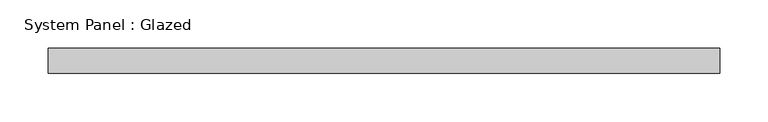
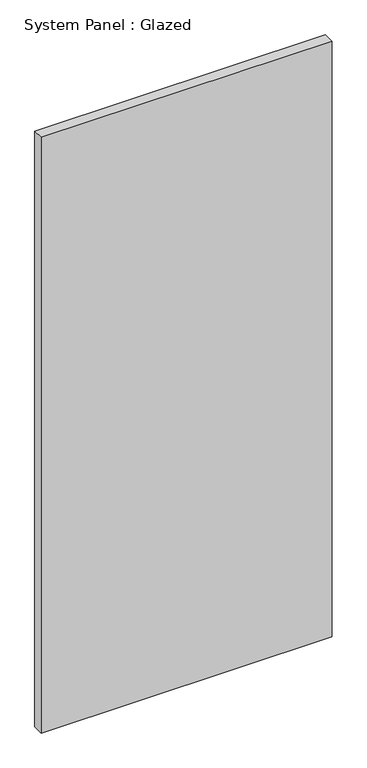
"""IFC4 building model written with IfcOpenShell, lengths in millimetres: plate geometry, System Panel : Glazed."""

from ifc_helpers import new_model, si_unit, origin, origin_with_axes, place, context, project, spatial, polyline, outline, extrude, source, transform, mapped, element, save


def system_panel_glazed_683b098e(model_context):
    return source(origin(), model_context, "Body", "SweptSolid", [
        extrude(outline(polyline([(346.075, 19.05), (-346.075, 19.05), (-346.075, 44.45), (346.075, 44.45), (346.075, 19.05)])), origin_with_axes(), (0.0, 0.0, 1.0), 1497.4964589),
    ])


if __name__ == "__main__":
    model = new_model("IFC4")
    model_context = context("Model", 3, world=origin())
    ifc_project = project(units=[si_unit("LENGTHUNIT", "METRE", prefix="MILLI")], contexts=[model_context])
    site = spatial("IfcSite", under=ifc_project)
    building = spatial("IfcBuilding", under=site)
    placement = place(None, origin())
    system_panel_glazed_shape = system_panel_glazed_683b098e(model_context)
    element("IfcPlate", 1, ObjectType="System Panel : Glazed", at=placement, inside=building, context=model_context, shape_type="MappedRepresentation", body=[
        mapped(system_panel_glazed_shape, transform((0.0, 0.0, 0.0), x_axis=(1.0, 0.0, 0.0), y_axis=(0.0, 1.0, 0.0), z_axis=(0.0, 0.0, 1.0))),
    ])
    save(model, "model.ifc")

# Revit data of these elements
# Type "System Panel : Glazed"
#   Construction Type Id = "GSP4R"
#   Analytic Construction = "1/8 in Pilkington single glazing"
#   Visual Light Transmittance = 0.9
#   Solar Heat Gain Coefficient = 0.86
#   Heat Transfer Coefficient (U) = 1.18115 BTU/(h·ft²·°F)
#   Define Thermal Properties by = 1
# Element 1 (IfcPlate, "System Panel : Glazed")
#   Materials on its faces: "Glass"
# Materials
#   "Glass": class "Glass", colour RGB 0 128 192, transparency 0.75, Description = "Soda Lime Glass", Cost = 0
